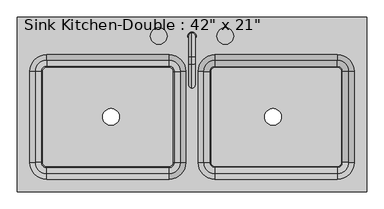
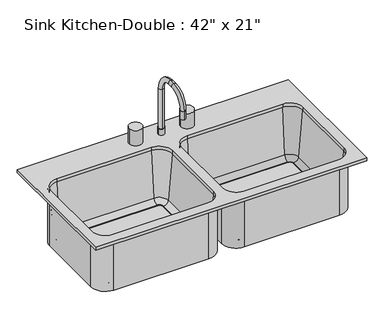
"""IFC4 building model written with IfcOpenShell, lengths in millimetres: flow terminal geometry."""

from ifc_helpers import new_model, si_unit, point, frame, frame_2d, origin, place, context, project, spatial, polyline, circle_curve, ellipse_curve, trimmed, segment, composite_curve, outline, extrude, source, transform, mapped, element, save
from ifc_brep_helpers import plane_surface, cylinder_surface, revolved_surface, advanced_brep


def flow_terminal_a53be723(model_context):
    return source(origin(), model_context, "Body", "SolidModel", [
        advanced_brep(
        [(2.9892406, 211.8954011, 927.1), (28.3892406, 211.8954011, 927.1), (15.6892406, 221.4204011, 1114.425), (15.6892406, 202.3704011, 1114.425), (15.6892406, 202.3704011, 952.5), (15.6892406, 221.4204011, 952.5), (15.6892406, 148.3954011, 1187.45), (15.6892406, 148.3954011, 1168.4), (15.6892406, 126.1704011, 1187.45), (15.6892406, 126.1704011, 1168.4), (15.6892406, 53.1454011, 1114.425), (15.6892406, 72.1954011, 1114.425), (15.6892406, 53.1454011, 1079.5), (15.6892406, 72.1954011, 1079.5), (2.9892406, 211.8954011, 952.5), (28.3892406, 211.8954011, 952.5)],
        [
            (0, 1, circle_curve(frame((15.6892406, 211.8954011, 927.1), z_axis=(0.0, 0.0, -1.0), x_axis=(1.0, 0.0, 0.0)), 12.7)),
            (1, 0, circle_curve(frame((15.6892406, 211.8954011, 927.1), z_axis=(0.0, 0.0, -1.0), x_axis=(1.0, 0.0, 0.0)), 12.7)),
            (2, 3, circle_curve(frame((15.6892406, 211.8954011, 1114.425), z_axis=(0.0, 0.0, -1.0), x_axis=(0.0, -1.0, 0.0)), 9.525)),
            (3, 4),
            (4, 5, circle_curve(frame((15.6892406, 211.8954011, 952.5), z_axis=(0.0, 0.0, 1.0), x_axis=(0.0, -1.0, 0.0)), 9.525)),
            (5, 2),
            (3, 2, circle_curve(frame((15.6892406, 211.8954011, 1114.425), z_axis=(0.0, 0.0, -1.0), x_axis=(0.0, -1.0, 0.0)), 9.525)),
            (5, 4, circle_curve(frame((15.6892406, 211.8954011, 952.5), z_axis=(0.0, 0.0, 1.0), x_axis=(0.0, -1.0, 0.0)), 9.525)),
            (2, 6, circle_curve(frame((15.6892406, 148.3954011, 1114.425), z_axis=(1.0, 0.0, 0.0), x_axis=(0.0, 1.0, 0.0)), 73.025)),
            (6, 7, circle_curve(frame((15.6892406, 148.3954011, 1177.925), z_axis=(0.0, 1.0, 0.0), x_axis=(0.0, 0.0, -1.0)), 9.525)),
            (7, 3, circle_curve(frame((15.6892406, 148.3954011, 1114.425), z_axis=(-1.0, 0.0, 0.0), x_axis=(0.0, 1.0, 0.0)), 53.975)),
            (7, 6, circle_curve(frame((15.6892406, 148.3954011, 1177.925), z_axis=(0.0, 1.0, 0.0), x_axis=(0.0, 0.0, -1.0)), 9.525)),
            (6, 8),
            (8, 9, circle_curve(frame((15.6892406, 126.1704011, 1177.925), z_axis=(0.0, 1.0, 0.0), x_axis=(0.0, 0.0, -1.0)), 9.525)),
            (9, 7),
            (9, 8, circle_curve(frame((15.6892406, 126.1704011, 1177.925), z_axis=(0.0, 1.0, 0.0), x_axis=(0.0, 0.0, -1.0)), 9.525)),
            (8, 10, circle_curve(frame((15.6892406, 126.1704011, 1114.425), z_axis=(1.0, 0.0, 0.0), x_axis=(0.0, 0.0, 1.0)), 73.025)),
            (10, 11, circle_curve(frame((15.6892406, 62.6704011, 1114.425), z_axis=(0.0, 0.0, 1.0), x_axis=(0.0, 1.0, 0.0)), 9.525)),
            (11, 9, circle_curve(frame((15.6892406, 126.1704011, 1114.425), z_axis=(-1.0, 0.0, 0.0), x_axis=(0.0, 0.0, 1.0)), 53.975)),
            (11, 10, circle_curve(frame((15.6892406, 62.6704011, 1114.425), z_axis=(0.0, 0.0, 1.0), x_axis=(0.0, 1.0, 0.0)), 9.525)),
            (12, 13, circle_curve(frame((15.6892406, 62.6704011, 1079.5), z_axis=(0.0, 0.0, -1.0), x_axis=(0.0, 1.0, 0.0)), 9.525)),
            (13, 12, circle_curve(frame((15.6892406, 62.6704011, 1079.5), z_axis=(0.0, 0.0, -1.0), x_axis=(0.0, 1.0, 0.0)), 9.525)),
            (10, 12),
            (13, 11),
            (14, 15, circle_curve(frame((15.6892406, 211.8954011, 952.5), z_axis=(0.0, 0.0, 1.0), x_axis=(1.0, 0.0, 0.0)), 12.7)),
            (15, 14, circle_curve(frame((15.6892406, 211.8954011, 952.5), z_axis=(0.0, 0.0, 1.0), x_axis=(1.0, 0.0, 0.0)), 12.7)),
            (14, 0),
            (1, 15),
        ],
        [
            plane_surface(frame((15.6892406, 202.3704011, 927.1), z_axis=(0.0, 0.0, -1.0), x_axis=(1.0, 0.0, 0.0))),
            cylinder_surface(frame((15.6892406, 211.8954011, 927.1), z_axis=(0.0, 0.0, -1.0), x_axis=(0.0, -1.0, 0.0)), 9.525),
            revolved_surface(trimmed(ellipse_curve(frame((15.6892406, 211.8954011, 1114.425), z_axis=(0.0, 0.0, -1.0), x_axis=(0.0, -1.0, 0.0)), 9.525, 9.525), [point((15.6892406, 221.4204011, 1114.425))], [point((15.6892406, 202.3704011, 1114.425))], True, "CARTESIAN"), (15.6892406, 148.3954011, 1114.425), (1.0, 0.0, 0.0)),
            revolved_surface(trimmed(ellipse_curve(frame((15.6892406, 211.8954011, 1114.425), z_axis=(0.0, 0.0, -1.0), x_axis=(0.0, -1.0, 0.0)), 9.525, 9.525), [point((15.6892406, 202.3704011, 1114.425))], [point((15.6892406, 221.4204011, 1114.425))], True, "CARTESIAN"), (15.6892406, 148.3954011, 1114.425), (1.0, 0.0, 0.0)),
            cylinder_surface(frame((15.6892406, 148.3954011, 1177.925), z_axis=(0.0, 1.0, 0.0), x_axis=(0.0, 0.0, -1.0)), 9.525),
            revolved_surface(trimmed(ellipse_curve(frame((15.6892406, 126.1704011, 1177.925), z_axis=(0.0, 1.0, 0.0), x_axis=(0.0, 0.0, -1.0)), 9.525, 9.525), [point((15.6892406, 126.1704011, 1187.45))], [point((15.6892406, 126.1704011, 1168.4))], True, "CARTESIAN"), (15.6892406, 126.1704011, 1114.425), (1.0, 0.0, 0.0)),
            revolved_surface(trimmed(ellipse_curve(frame((15.6892406, 126.1704011, 1177.925), z_axis=(0.0, 1.0, 0.0), x_axis=(0.0, 0.0, -1.0)), 9.525, 9.525), [point((15.6892406, 126.1704011, 1168.4))], [point((15.6892406, 126.1704011, 1187.45))], True, "CARTESIAN"), (15.6892406, 126.1704011, 1114.425), (1.0, 0.0, 0.0)),
            plane_surface(frame((15.6892406, 53.1454011, 1079.5), z_axis=(0.0, 0.0, -1.0), x_axis=(-1.0, 0.0, 0.0))),
            cylinder_surface(frame((15.6892406, 62.6704011, 1114.425), z_axis=(0.0, 0.0, 1.0), x_axis=(0.0, 1.0, 0.0)), 9.525),
            plane_surface(frame((28.3892406, 211.8954011, 952.5), z_axis=(0.0, 0.0, 1.0), x_axis=(0.0, 1.0, 0.0))),
            cylinder_surface(frame((15.6892406, 211.8954011, 927.1), z_axis=(0.0, 0.0, 1.0), x_axis=(1.0, 0.0, 0.0)), 12.7),
        ],
        [
            (0, [[1, 2]]),
            (1, [[3, 4, 5, 6]]),
            (1, [[7, -6, 8, -4]]),
            (2, [[-3, 9, 10, 11]]),
            (3, [[-7, -11, 12, -9]]),
            (4, [[-10, 13, 14, 15]]),
            (4, [[-12, -15, 16, -13]]),
            (5, [[-14, 17, 18, 19]]),
            (6, [[-16, -19, 20, -17]]),
            (7, [[21, 22]]),
            (8, [[-18, 23, -22, 24]]),
            (8, [[-20, -24, -21, -23]]),
            (9, [[25, 26], [-5, -8]]),
            (10, [[-25, 27, -2, 28]]),
            (10, [[-26, -28, -1, -27]]),
        ],
    ),
        advanced_brep(
        [(549.0892406, 269.0454011, 927.1), (-517.7107594, 269.0454011, 927.1), (-517.7107594, -264.3545989, 927.1), (549.0892406, -264.3545989, 927.1), (-54.1607594, 154.7454011, 927.1), (-3.3607594, 103.9454011, 927.1), (-3.3607594, -175.4545989, 927.1), (-54.1607594, -226.2545989, 927.1), (-428.8107594, -226.2545989, 927.1), (-479.6107594, -175.4545989, 927.1), (-479.6107594, 103.9454011, 927.1), (-428.8107594, 154.7454011, 927.1), (85.5392406, -226.2545989, 927.1), (34.7392406, -175.4545989, 927.1), (34.7392406, 103.9454011, 927.1), (85.5392406, 154.7454011, 927.1), (460.1892406, 154.7454011, 927.1), (510.9892406, 103.9454011, 927.1), (510.9892406, -175.4545989, 927.1), (460.1892406, -226.2545989, 927.1), (549.0892406, 269.0454011, 914.4), (549.0892406, -264.3545989, 914.4), (-517.7107594, -264.3545989, 914.4), (-517.7107594, 269.0454011, 914.4), (85.5392406, 161.0954011, 914.4), (28.3892406, 103.9454011, 914.4), (28.3892406, -175.4545989, 914.4), (85.5392406, -232.6045989, 914.4), (460.1892406, -232.6045989, 914.4), (517.3392406, -175.4545989, 914.4), (517.3392406, 103.9454011, 914.4), (460.1892406, 161.0954011, 914.4), (2.9892406, 103.9454011, 914.4), (-54.1607594, 161.0954011, 914.4), (-428.8107594, 161.0954011, 914.4), (-485.9607594, 103.9454011, 914.4), (-485.9607594, -175.4545989, 914.4), (-428.8107594, -232.6045989, 914.4), (-54.1607594, -232.6045989, 914.4), (2.9892406, -175.4545989, 914.4), (-54.1607594, 154.7454011, 914.4), (-3.3607594, 103.9454011, 914.4), (-3.3607594, -175.4545989, 914.4), (-54.1607594, -226.2545989, 914.4), (-428.8107594, -226.2545989, 914.4), (-479.6107594, -175.4545989, 914.4), (-479.6107594, 103.9454011, 914.4), (-428.8107594, 154.7454011, 914.4), (85.5392406, -226.2545989, 914.4), (34.7392406, -175.4545989, 914.4), (34.7392406, 103.9454011, 914.4), (85.5392406, 154.7454011, 914.4), (460.1892406, 154.7454011, 914.4), (510.9892406, 103.9454011, 914.4), (510.9892406, -175.4545989, 914.4), (460.1892406, -226.2545989, 914.4), (51.2733134, 103.9454011, 725.4146831), (85.5392406, 138.2113283, 725.4146831), (70.2508224, 103.9454011, 708.025), (85.5392406, 119.2338193, 708.025), (72.8392406, 103.9454011, 708.025), (85.5392406, 116.6454011, 708.025), (72.8392406, 103.9454011, 698.5), (85.5392406, 116.6454011, 698.5), (28.3892406, 103.9454011, 698.5), (85.5392406, 161.0954011, 698.5), (51.2733134, -175.4545989, 725.4146831), (70.2508224, -175.4545989, 708.025), (72.8392406, -175.4545989, 708.025), (72.8392406, -175.4545989, 698.5), (28.3892406, -175.4545989, 698.5), (85.5392406, -209.7205261, 725.4146831), (85.5392406, -190.7430171, 708.025), (85.5392406, -188.1545989, 708.025), (85.5392406, -188.1545989, 698.5), (85.5392406, -232.6045989, 698.5), (460.1892406, -209.7205261, 725.4146831), (460.1892406, -190.7430171, 708.025), (460.1892406, -188.1545989, 708.025), (460.1892406, -188.1545989, 698.5), (460.1892406, -232.6045989, 698.5), (494.4551678, -175.4545989, 725.4146831), (475.4776588, -175.4545989, 708.025), (472.8892406, -175.4545989, 708.025), (472.8892406, -175.4545989, 698.5), (517.3392406, -175.4545989, 698.5), (494.4551678, 103.9454011, 725.4146831), (475.4776588, 103.9454011, 708.025), (472.8892406, 103.9454011, 708.025), (472.8892406, 103.9454011, 698.5), (517.3392406, 103.9454011, 698.5), (460.1892406, 138.2113283, 725.4146831), (460.1892406, 119.2338193, 708.025), (460.1892406, 116.6454011, 708.025), (460.1892406, 116.6454011, 698.5), (460.1892406, 161.0954011, 698.5), (2.9892406, 103.9454011, 698.5), (-54.1607594, 161.0954011, 698.5), (-41.4607594, 103.9454011, 698.5), (-54.1607594, 116.6454011, 698.5), (-41.4607594, 103.9454011, 708.025), (-54.1607594, 116.6454011, 708.025), (-38.8723412, 103.9454011, 708.025), (-54.1607594, 119.2338193, 708.025), (-19.8948322, 103.9454011, 725.4146831), (-54.1607594, 138.2113283, 725.4146831), (2.9892406, -175.4545989, 698.5), (-41.4607594, -175.4545989, 698.5), (-41.4607594, -175.4545989, 708.025), (-38.8723412, -175.4545989, 708.025), (-19.8948322, -175.4545989, 725.4146831), (-54.1607594, -232.6045989, 698.5), (-54.1607594, -188.1545989, 698.5), (-54.1607594, -188.1545989, 708.025), (-54.1607594, -190.7430171, 708.025), (-54.1607594, -209.7205261, 725.4146831), (-428.8107594, -232.6045989, 698.5), (-428.8107594, -188.1545989, 698.5), (-428.8107594, -188.1545989, 708.025), (-428.8107594, -190.7430171, 708.025), (-428.8107594, -209.7205261, 725.4146831), (-485.9607594, -175.4545989, 698.5), (-441.5107594, -175.4545989, 698.5), (-441.5107594, -175.4545989, 708.025), (-444.0991776, -175.4545989, 708.025), (-463.0766866, -175.4545989, 725.4146831), (-485.9607594, 103.9454011, 698.5), (-441.5107594, 103.9454011, 698.5), (-441.5107594, 103.9454011, 708.025), (-444.0991776, 103.9454011, 708.025), (-463.0766866, 103.9454011, 725.4146831), (-428.8107594, 161.0954011, 698.5), (-428.8107594, 116.6454011, 698.5), (-428.8107594, 116.6454011, 708.025), (-428.8107594, 119.2338193, 708.025), (-428.8107594, 138.2113283, 725.4146831)],
        [
            (0, 1),
            (1, 2),
            (2, 3),
            (3, 0),
            (4, 5, circle_curve(frame((-54.1607594, 103.9454011, 927.1), z_axis=(0.0, 0.0, -1.0), x_axis=(1.0, 0.0, 0.0)), 50.8)),
            (5, 6),
            (6, 7, circle_curve(frame((-54.1607594, -175.4545989, 927.1), z_axis=(0.0, 0.0, -1.0), x_axis=(1.0, 0.0, 0.0)), 50.8)),
            (7, 8),
            (8, 9, circle_curve(frame((-428.8107594, -175.4545989, 927.1), z_axis=(0.0, 0.0, -1.0), x_axis=(1.0, 0.0, 0.0)), 50.8)),
            (9, 10),
            (10, 11, circle_curve(frame((-428.8107594, 103.9454011, 927.1), z_axis=(0.0, 0.0, -1.0), x_axis=(1.0, 0.0, 0.0)), 50.8)),
            (11, 4),
            (12, 13, circle_curve(frame((85.5392406, -175.4545989, 927.1), z_axis=(0.0, 0.0, -1.0), x_axis=(1.0, 0.0, 0.0)), 50.8)),
            (13, 14),
            (14, 15, circle_curve(frame((85.5392406, 103.9454011, 927.1), z_axis=(0.0, 0.0, -1.0), x_axis=(1.0, 0.0, 0.0)), 50.8)),
            (15, 16),
            (16, 17, circle_curve(frame((460.1892406, 103.9454011, 927.1), z_axis=(0.0, 0.0, -1.0), x_axis=(1.0, 0.0, 0.0)), 50.8)),
            (17, 18),
            (18, 19, circle_curve(frame((460.1892406, -175.4545989, 927.1), z_axis=(0.0, 0.0, -1.0), x_axis=(1.0, 0.0, 0.0)), 50.8)),
            (19, 12),
            (20, 21),
            (21, 22),
            (22, 23),
            (23, 20),
            (24, 25, circle_curve(frame((85.5392406, 103.9454011, 914.4), z_axis=(0.0, 0.0, 1.0), x_axis=(0.0, 1.0, 0.0)), 57.15)),
            (25, 26),
            (26, 27, circle_curve(frame((85.5392406, -175.4545989, 914.4), z_axis=(0.0, 0.0, 1.0), x_axis=(-1.0, 0.0, 0.0)), 57.15)),
            (27, 28),
            (28, 29, circle_curve(frame((460.1892406, -175.4545989, 914.4), z_axis=(0.0, 0.0, 1.0), x_axis=(0.0, -1.0, 0.0)), 57.15)),
            (29, 30),
            (30, 31, circle_curve(frame((460.1892406, 103.9454011, 914.4), z_axis=(0.0, 0.0, 1.0), x_axis=(1.0, 0.0, 0.0)), 57.15)),
            (31, 24),
            (32, 33, circle_curve(frame((-54.1607594, 103.9454011, 914.4), z_axis=(0.0, 0.0, 1.0), x_axis=(0.0, 1.0, 0.0)), 57.15)),
            (33, 34),
            (34, 35, circle_curve(frame((-428.8107594, 103.9454011, 914.4), z_axis=(0.0, 0.0, 1.0), x_axis=(-1.0, 0.0, 0.0)), 57.15)),
            (35, 36),
            (36, 37, circle_curve(frame((-428.8107594, -175.4545989, 914.4), z_axis=(0.0, 0.0, 1.0), x_axis=(0.0, -1.0, 0.0)), 57.15)),
            (37, 38),
            (38, 39, circle_curve(frame((-54.1607594, -175.4545989, 914.4), z_axis=(0.0, 0.0, 1.0), x_axis=(1.0, 0.0, 0.0)), 57.15)),
            (39, 32),
            (0, 20),
            (23, 1),
            (22, 2),
            (21, 3),
            (4, 40),
            (40, 41, circle_curve(frame((-54.1607594, 103.9454011, 914.4), z_axis=(0.0, 0.0, -1.0), x_axis=(1.0, 0.0, 0.0)), 50.8)),
            (41, 5),
            (41, 42),
            (42, 6),
            (42, 43, circle_curve(frame((-54.1607594, -175.4545989, 914.4), z_axis=(0.0, 0.0, -1.0), x_axis=(1.0, 0.0, 0.0)), 50.8)),
            (43, 7),
            (43, 44),
            (44, 8),
            (44, 45, circle_curve(frame((-428.8107594, -175.4545989, 914.4), z_axis=(0.0, 0.0, -1.0), x_axis=(1.0, 0.0, 0.0)), 50.8)),
            (45, 9),
            (45, 46),
            (46, 10),
            (46, 47, circle_curve(frame((-428.8107594, 103.9454011, 914.4), z_axis=(0.0, 0.0, -1.0), x_axis=(1.0, 0.0, 0.0)), 50.8)),
            (47, 11),
            (47, 40),
            (12, 48),
            (48, 49, circle_curve(frame((85.5392406, -175.4545989, 914.4), z_axis=(0.0, 0.0, -1.0), x_axis=(1.0, 0.0, 0.0)), 50.8)),
            (49, 13),
            (49, 50),
            (50, 14),
            (50, 51, circle_curve(frame((85.5392406, 103.9454011, 914.4), z_axis=(0.0, 0.0, -1.0), x_axis=(1.0, 0.0, 0.0)), 50.8)),
            (51, 15),
            (51, 52),
            (52, 16),
            (52, 53, circle_curve(frame((460.1892406, 103.9454011, 914.4), z_axis=(0.0, 0.0, -1.0), x_axis=(1.0, 0.0, 0.0)), 50.8)),
            (53, 17),
            (53, 54),
            (54, 18),
            (54, 55, circle_curve(frame((460.1892406, -175.4545989, 914.4), z_axis=(0.0, 0.0, -1.0), x_axis=(1.0, 0.0, 0.0)), 50.8)),
            (55, 19),
            (55, 48),
            (56, 57, circle_curve(frame((85.5392406, 103.9454011, 725.4146831), z_axis=(0.0, 0.0, -1.0), x_axis=(0.0, 1.0, 0.0)), 34.2659272)),
            (57, 51),
            (50, 56),
            (56, 58, circle_curve(frame((70.2508224, 103.9454011, 727.075), z_axis=(0.0, -1.0, 0.0), x_axis=(1.0, 0.0, 0.0)), 19.05)),
            (58, 59, circle_curve(frame((85.5392406, 103.9454011, 708.025), z_axis=(0.0, 0.0, -1.0), x_axis=(0.0, 1.0, 0.0)), 15.2884182)),
            (59, 57, circle_curve(frame((85.5392406, 119.2338193, 727.075), z_axis=(1.0, 0.0, 0.0), x_axis=(0.0, -1.0, 0.0)), 19.05)),
            (58, 60),
            (60, 61, circle_curve(frame((85.5392406, 103.9454011, 708.025), z_axis=(0.0, 0.0, -1.0), x_axis=(0.0, 1.0, 0.0)), 12.7)),
            (61, 59),
            (60, 62),
            (62, 63, circle_curve(frame((85.5392406, 103.9454011, 698.5), z_axis=(0.0, 0.0, -1.0), x_axis=(0.0, 1.0, 0.0)), 12.7)),
            (63, 61),
            (62, 64),
            (64, 65, circle_curve(frame((85.5392406, 103.9454011, 698.5), z_axis=(0.0, 0.0, -1.0), x_axis=(0.0, 1.0, 0.0)), 57.15)),
            (65, 63),
            (64, 25),
            (24, 65),
            (49, 66),
            (66, 56),
            (66, 67, circle_curve(frame((70.2508224, -175.4545989, 727.075), z_axis=(0.0, -1.0, 0.0), x_axis=(1.0, 0.0, 0.0)), 19.05)),
            (67, 58),
            (67, 68),
            (68, 60),
            (68, 69),
            (69, 62),
            (69, 70),
            (70, 64),
            (70, 26),
            (48, 71),
            (71, 66, circle_curve(frame((85.5392406, -175.4545989, 725.4146831), z_axis=(0.0, 0.0, -1.0), x_axis=(-1.0, 0.0, 0.0)), 34.2659272)),
            (71, 72, circle_curve(frame((85.5392406, -190.7430171, 727.075), z_axis=(1.0, 0.0, 0.0), x_axis=(0.0, 1.0, 0.0)), 19.05)),
            (72, 67, circle_curve(frame((85.5392406, -175.4545989, 708.025), z_axis=(0.0, 0.0, -1.0), x_axis=(-1.0, 0.0, 0.0)), 15.2884182)),
            (72, 73),
            (73, 68, circle_curve(frame((85.5392406, -175.4545989, 708.025), z_axis=(0.0, 0.0, -1.0), x_axis=(-1.0, 0.0, 0.0)), 12.7)),
            (73, 74),
            (74, 69, circle_curve(frame((85.5392406, -175.4545989, 698.5), z_axis=(0.0, 0.0, -1.0), x_axis=(-1.0, 0.0, 0.0)), 12.7)),
            (74, 75),
            (75, 70, circle_curve(frame((85.5392406, -175.4545989, 698.5), z_axis=(0.0, 0.0, -1.0), x_axis=(-1.0, 0.0, 0.0)), 57.15)),
            (75, 27),
            (55, 76),
            (76, 71),
            (76, 77, circle_curve(frame((460.1892406, -190.7430171, 727.075), z_axis=(1.0, 0.0, 0.0), x_axis=(0.0, 1.0, 0.0)), 19.05)),
            (77, 72),
            (77, 78),
            (78, 73),
            (78, 79),
            (79, 74),
            (79, 80),
            (80, 75),
            (80, 28),
            (54, 81),
            (81, 76, circle_curve(frame((460.1892406, -175.4545989, 725.4146831), z_axis=(0.0, 0.0, -1.0), x_axis=(0.0, -1.0, 0.0)), 34.2659272)),
            (81, 82, circle_curve(frame((475.4776588, -175.4545989, 727.075), z_axis=(0.0, 1.0, 0.0), x_axis=(-1.0, 0.0, 0.0)), 19.05)),
            (82, 77, circle_curve(frame((460.1892406, -175.4545989, 708.025), z_axis=(0.0, 0.0, -1.0), x_axis=(0.0, -1.0, 0.0)), 15.2884182)),
            (82, 83),
            (83, 78, circle_curve(frame((460.1892406, -175.4545989, 708.025), z_axis=(0.0, 0.0, -1.0), x_axis=(0.0, -1.0, 0.0)), 12.7)),
            (83, 84),
            (84, 79, circle_curve(frame((460.1892406, -175.4545989, 698.5), z_axis=(0.0, 0.0, -1.0), x_axis=(0.0, -1.0, 0.0)), 12.7)),
            (84, 85),
            (85, 80, circle_curve(frame((460.1892406, -175.4545989, 698.5), z_axis=(0.0, 0.0, -1.0), x_axis=(0.0, -1.0, 0.0)), 57.15)),
            (85, 29),
            (53, 86),
            (86, 81),
            (86, 87, circle_curve(frame((475.4776588, 103.9454011, 727.075), z_axis=(0.0, 1.0, 0.0), x_axis=(-1.0, 0.0, 0.0)), 19.05)),
            (87, 82),
            (87, 88),
            (88, 83),
            (88, 89),
            (89, 84),
            (89, 90),
            (90, 85),
            (90, 30),
            (52, 91),
            (91, 86, circle_curve(frame((460.1892406, 103.9454011, 725.4146831), z_axis=(0.0, 0.0, -1.0), x_axis=(1.0, 0.0, 0.0)), 34.2659272)),
            (91, 92, circle_curve(frame((460.1892406, 119.2338193, 727.075), z_axis=(-1.0, 0.0, 0.0), x_axis=(0.0, -1.0, 0.0)), 19.05)),
            (92, 87, circle_curve(frame((460.1892406, 103.9454011, 708.025), z_axis=(0.0, 0.0, -1.0), x_axis=(1.0, 0.0, 0.0)), 15.2884182)),
            (92, 93),
            (93, 88, circle_curve(frame((460.1892406, 103.9454011, 708.025), z_axis=(0.0, 0.0, -1.0), x_axis=(1.0, 0.0, 0.0)), 12.7)),
            (93, 94),
            (94, 89, circle_curve(frame((460.1892406, 103.9454011, 698.5), z_axis=(0.0, 0.0, -1.0), x_axis=(1.0, 0.0, 0.0)), 12.7)),
            (94, 95),
            (95, 90, circle_curve(frame((460.1892406, 103.9454011, 698.5), z_axis=(0.0, 0.0, -1.0), x_axis=(1.0, 0.0, 0.0)), 57.15)),
            (95, 31),
            (57, 91),
            (59, 92),
            (61, 93),
            (63, 94),
            (65, 95),
            (96, 97, circle_curve(frame((-54.1607594, 103.9454011, 698.5), z_axis=(0.0, 0.0, 1.0), x_axis=(0.0, 1.0, 0.0)), 57.15)),
            (97, 33),
            (32, 96),
            (96, 98),
            (98, 99, circle_curve(frame((-54.1607594, 103.9454011, 698.5), z_axis=(0.0, 0.0, 1.0), x_axis=(0.0, 1.0, 0.0)), 12.7)),
            (99, 97),
            (98, 100),
            (100, 101, circle_curve(frame((-54.1607594, 103.9454011, 708.025), z_axis=(0.0, 0.0, 1.0), x_axis=(0.0, 1.0, 0.0)), 12.7)),
            (101, 99),
            (100, 102),
            (102, 103, circle_curve(frame((-54.1607594, 103.9454011, 708.025), z_axis=(0.0, 0.0, 1.0), x_axis=(0.0, 1.0, 0.0)), 15.2884182)),
            (103, 101),
            (102, 104, circle_curve(frame((-38.8723412, 103.9454011, 727.075), z_axis=(0.0, -1.0, 0.0), x_axis=(1.0, 0.0, 0.0)), 19.05)),
            (104, 105, circle_curve(frame((-54.1607594, 103.9454011, 725.4146831), z_axis=(0.0, 0.0, 1.0), x_axis=(0.0, 1.0, 0.0)), 34.2659272)),
            (105, 103, circle_curve(frame((-54.1607594, 119.2338193, 727.075), z_axis=(-1.0, 0.0, 0.0), x_axis=(0.0, 1.0, 0.0)), 19.05)),
            (104, 41),
            (40, 105),
            (39, 106),
            (106, 96),
            (106, 107),
            (107, 98),
            (107, 108),
            (108, 100),
            (108, 109),
            (109, 102),
            (109, 110, circle_curve(frame((-38.8723412, -175.4545989, 727.075), z_axis=(0.0, -1.0, 0.0), x_axis=(1.0, 0.0, 0.0)), 19.05)),
            (110, 104),
            (110, 42),
            (38, 111),
            (111, 106, circle_curve(frame((-54.1607594, -175.4545989, 698.5), z_axis=(0.0, 0.0, 1.0), x_axis=(1.0, 0.0, 0.0)), 57.15)),
            (111, 112),
            (112, 107, circle_curve(frame((-54.1607594, -175.4545989, 698.5), z_axis=(0.0, 0.0, 1.0), x_axis=(1.0, 0.0, 0.0)), 12.7)),
            (112, 113),
            (113, 108, circle_curve(frame((-54.1607594, -175.4545989, 708.025), z_axis=(0.0, 0.0, 1.0), x_axis=(1.0, 0.0, 0.0)), 12.7)),
            (113, 114),
            (114, 109, circle_curve(frame((-54.1607594, -175.4545989, 708.025), z_axis=(0.0, 0.0, 1.0), x_axis=(1.0, 0.0, 0.0)), 15.2884182)),
            (114, 115, circle_curve(frame((-54.1607594, -190.7430171, 727.075), z_axis=(-1.0, 0.0, 0.0), x_axis=(0.0, -1.0, 0.0)), 19.05)),
            (115, 110, circle_curve(frame((-54.1607594, -175.4545989, 725.4146831), z_axis=(0.0, 0.0, 1.0), x_axis=(1.0, 0.0, 0.0)), 34.2659272)),
            (115, 43),
            (37, 116),
            (116, 111),
            (116, 117),
            (117, 112),
            (117, 118),
            (118, 113),
            (118, 119),
            (119, 114),
            (119, 120, circle_curve(frame((-428.8107594, -190.7430171, 727.075), z_axis=(-1.0, 0.0, 0.0), x_axis=(0.0, -1.0, 0.0)), 19.05)),
            (120, 115),
            (120, 44),
            (36, 121),
            (121, 116, circle_curve(frame((-428.8107594, -175.4545989, 698.5), z_axis=(0.0, 0.0, 1.0), x_axis=(0.0, -1.0, 0.0)), 57.15)),
            (121, 122),
            (122, 117, circle_curve(frame((-428.8107594, -175.4545989, 698.5), z_axis=(0.0, 0.0, 1.0), x_axis=(0.0, -1.0, 0.0)), 12.7)),
            (122, 123),
            (123, 118, circle_curve(frame((-428.8107594, -175.4545989, 708.025), z_axis=(0.0, 0.0, 1.0), x_axis=(0.0, -1.0, 0.0)), 12.7)),
            (123, 124),
            (124, 119, circle_curve(frame((-428.8107594, -175.4545989, 708.025), z_axis=(0.0, 0.0, 1.0), x_axis=(0.0, -1.0, 0.0)), 15.2884182)),
            (124, 125, circle_curve(frame((-444.0991776, -175.4545989, 727.075), z_axis=(0.0, 1.0, 0.0), x_axis=(-1.0, 0.0, 0.0)), 19.05)),
            (125, 120, circle_curve(frame((-428.8107594, -175.4545989, 725.4146831), z_axis=(0.0, 0.0, 1.0), x_axis=(0.0, -1.0, 0.0)), 34.2659272)),
            (125, 45),
            (35, 126),
            (126, 121),
            (126, 127),
            (127, 122),
            (127, 128),
            (128, 123),
            (128, 129),
            (129, 124),
            (129, 130, circle_curve(frame((-444.0991776, 103.9454011, 727.075), z_axis=(0.0, 1.0, 0.0), x_axis=(-1.0, 0.0, 0.0)), 19.05)),
            (130, 125),
            (130, 46),
            (34, 131),
            (131, 126, circle_curve(frame((-428.8107594, 103.9454011, 698.5), z_axis=(0.0, 0.0, 1.0), x_axis=(-1.0, 0.0, 0.0)), 57.15)),
            (131, 132),
            (132, 127, circle_curve(frame((-428.8107594, 103.9454011, 698.5), z_axis=(0.0, 0.0, 1.0), x_axis=(-1.0, 0.0, 0.0)), 12.7)),
            (132, 133),
            (133, 128, circle_curve(frame((-428.8107594, 103.9454011, 708.025), z_axis=(0.0, 0.0, 1.0), x_axis=(-1.0, 0.0, 0.0)), 12.7)),
            (133, 134),
            (134, 129, circle_curve(frame((-428.8107594, 103.9454011, 708.025), z_axis=(0.0, 0.0, 1.0), x_axis=(-1.0, 0.0, 0.0)), 15.2884182)),
            (134, 135, circle_curve(frame((-428.8107594, 119.2338193, 727.075), z_axis=(1.0, 0.0, 0.0), x_axis=(0.0, 1.0, 0.0)), 19.05)),
            (135, 130, circle_curve(frame((-428.8107594, 103.9454011, 725.4146831), z_axis=(0.0, 0.0, 1.0), x_axis=(-1.0, 0.0, 0.0)), 34.2659272)),
            (135, 47),
            (97, 131),
            (99, 132),
            (101, 133),
            (103, 134),
            (105, 135),
        ],
        [
            plane_surface(frame((-517.7107594, 269.0454011, 927.1), z_axis=(0.0, 0.0, 1.0), x_axis=(-1.0, 0.0, 0.0))),
            plane_surface(frame((-517.7107594, 269.0454011, 914.4), z_axis=(0.0, 0.0, -1.0), x_axis=(1.0, 0.0, 0.0))),
            plane_surface(frame((549.0892406, 269.0454011, 927.1), z_axis=(0.0, 1.0, 0.0), x_axis=(0.0, 0.0, -1.0))),
            plane_surface(frame((-517.7107594, 269.0454011, 927.1), z_axis=(-1.0, 0.0, 0.0), x_axis=(0.0, 0.0, -1.0))),
            plane_surface(frame((-517.7107594, -264.3545989, 927.1), z_axis=(0.0, -1.0, 0.0), x_axis=(0.0, 0.0, -1.0))),
            plane_surface(frame((549.0892406, -264.3545989, 927.1), z_axis=(1.0, 0.0, 0.0), x_axis=(0.0, 0.0, -1.0))),
            revolved_surface(polyline([(-3.3607594000000063, 103.9454011, 914.4), (-3.3607594000000063, 103.9454011, 927.1)]), (-54.1607594, 103.9454011, 0.0), (0.0, 0.0, -1.0)),
            plane_surface(frame((-3.3607594, 103.9454011, 927.1), z_axis=(-1.0, 0.0, 0.0), x_axis=(0.0, 0.0, -1.0))),
            revolved_surface(polyline([(-3.3607594000000063, -175.4545989, 914.4), (-3.3607594000000063, -175.4545989, 927.1)]), (-54.1607594, -175.4545989, 0.0), (0.0, 0.0, -1.0)),
            plane_surface(frame((-54.1607594, -226.2545989, 927.1), z_axis=(0.0, 1.0, 0.0), x_axis=(0.0, 0.0, -1.0))),
            revolved_surface(polyline([(-378.0107594, -175.4545989, 914.4), (-378.0107594, -175.4545989, 927.1)]), (-428.8107594, -175.4545989, 0.0), (0.0, 0.0, -1.0)),
            plane_surface(frame((-479.6107594, -175.4545989, 927.1), z_axis=(1.0, 0.0, 0.0), x_axis=(0.0, 0.0, -1.0))),
            revolved_surface(polyline([(-378.0107594, 103.9454011, 914.4), (-378.0107594, 103.9454011, 927.1)]), (-428.8107594, 103.9454011, 0.0), (0.0, 0.0, -1.0)),
            plane_surface(frame((-428.8107594, 154.7454011, 927.1), z_axis=(0.0, -1.0, 0.0), x_axis=(0.0, 0.0, -1.0))),
            revolved_surface(polyline([(136.33924059999998, -175.4545989, 914.4), (136.33924059999998, -175.4545989, 927.1)]), (85.5392406, -175.4545989, 0.0), (0.0, 0.0, -1.0)),
            plane_surface(frame((34.7392406, -175.4545989, 927.1), z_axis=(1.0, 0.0, 0.0), x_axis=(0.0, 0.0, -1.0))),
            revolved_surface(polyline([(136.33924059999998, 103.9454011, 914.4), (136.33924059999998, 103.9454011, 927.1)]), (85.5392406, 103.9454011, 0.0), (0.0, 0.0, -1.0)),
            plane_surface(frame((85.5392406, 154.7454011, 927.1), z_axis=(0.0, -1.0, 0.0), x_axis=(0.0, 0.0, -1.0))),
            revolved_surface(polyline([(510.9892406, 103.9454011, 914.4), (510.9892406, 103.9454011, 927.1)]), (460.1892406, 103.9454011, 0.0), (0.0, 0.0, -1.0)),
            plane_surface(frame((510.9892406, 103.9454011, 927.1), z_axis=(-1.0, 0.0, 0.0), x_axis=(0.0, 0.0, -1.0))),
            revolved_surface(polyline([(510.9892406, -175.4545989, 914.4), (510.9892406, -175.4545989, 927.1)]), (460.1892406, -175.4545989, 0.0), (0.0, 0.0, -1.0)),
            plane_surface(frame((460.1892406, -226.2545989, 927.1), z_axis=(0.0, 1.0, 0.0), x_axis=(0.0, 0.0, -1.0))),
            revolved_surface(polyline([(85.5392406, 154.7454011, 914.4), (85.5392406, 138.2113283, 725.4146831)]), (85.5392406, 103.9454011, 0.0), (0.0, 0.0, 1.0)),
            revolved_surface(trimmed(ellipse_curve(frame((85.5392406, 119.2338193, 727.075), z_axis=(-1.0, 0.0, 0.0), x_axis=(0.0, -1.0, 0.0)), 19.05, 19.05), [point((85.5392406, 138.2113283, 725.4146831))], [point((85.5392406, 119.2338193, 708.025))], True, "CARTESIAN"), (85.5392406, 103.9454011, 0.0), (0.0, 0.0, 1.0)),
            plane_surface(frame((85.5392406, 103.9454011, 708.025), z_axis=(0.0, 0.0, 1.0), x_axis=(0.0, 1.0, 0.0))),
            revolved_surface(polyline([(85.5392406, 116.6454011, 708.025), (85.5392406, 116.6454011, 698.5)]), (85.5392406, 103.9454011, 0.0), (0.0, 0.0, 1.0)),
            plane_surface(frame((85.5392406, 103.9454011, 698.5), z_axis=(0.0, 0.0, -1.0), x_axis=(0.0, 1.0, 0.0))),
            cylinder_surface(frame((85.5392406, 103.9454011, 0.0), z_axis=(0.0, 0.0, 1.0), x_axis=(0.0, 1.0, 0.0)), 57.15),
            plane_surface(frame((34.7392406, 103.9454011, 914.4), z_axis=(0.996194698091745, 0.0, 0.08715574274766508), x_axis=(0.0, -1.0, 0.0))),
            revolved_surface(polyline([(89.3008224, -175.45459889999998, 727.075), (89.3008224, 103.9454011, 727.075)]), (70.2508224, 103.9454011, 727.075), (0.0, -1.0, 0.0)),
            plane_surface(frame((70.2508224, 103.9454011, 708.025), z_axis=(0.0, 0.0, 1.0), x_axis=(0.0, -1.0, 0.0))),
            plane_surface(frame((72.8392406, 103.9454011, 708.025), z_axis=(1.0, 0.0, 0.0), x_axis=(0.0, -1.0, 0.0))),
            plane_surface(frame((72.8392406, 103.9454011, 698.5), z_axis=(0.0, 0.0, -1.0), x_axis=(0.0, -1.0, 0.0))),
            plane_surface(frame((28.3892406, 103.9454011, 698.5), z_axis=(-1.0, 0.0, 0.0), x_axis=(0.0, -1.0, 0.0))),
            revolved_surface(polyline([(34.7392406, -175.4545989, 914.4), (51.2733134, -175.4545989, 725.4146831)]), (85.5392406, -175.4545989, 0.0), (0.0, 0.0, 1.0)),
            revolved_surface(trimmed(ellipse_curve(frame((70.2508224, -175.4545989, 727.075), z_axis=(0.0, -1.0, 0.0), x_axis=(1.0, 0.0, 0.0)), 19.05, 19.05), [point((51.2733134, -175.4545989, 725.4146831))], [point((70.2508224, -175.4545989, 708.025))], True, "CARTESIAN"), (85.5392406, -175.4545989, 0.0), (0.0, 0.0, 1.0)),
            plane_surface(frame((85.5392406, -175.4545989, 708.025), z_axis=(0.0, 0.0, 1.0), x_axis=(-1.0, 0.0, 0.0))),
            revolved_surface(polyline([(72.8392406, -175.4545989, 708.025), (72.8392406, -175.4545989, 698.5)]), (85.5392406, -175.4545989, 0.0), (0.0, 0.0, 1.0)),
            plane_surface(frame((85.5392406, -175.4545989, 698.5), z_axis=(0.0, 0.0, -1.0), x_axis=(-1.0, 0.0, 0.0))),
            cylinder_surface(frame((85.5392406, -175.4545989, 0.0), z_axis=(0.0, 0.0, 1.0), x_axis=(-1.0, 0.0, 0.0)), 57.15),
            plane_surface(frame((85.5392406, -226.2545989, 914.4), z_axis=(0.0, 0.996194698091745, 0.08715574274766508), x_axis=(1.0, 0.0, 0.0))),
            revolved_surface(polyline([(460.18924059999995, -171.6930171, 727.075), (85.5392406, -171.6930171, 727.075)]), (85.5392406, -190.7430171, 727.075), (1.0, 0.0, 0.0)),
            plane_surface(frame((85.5392406, -190.7430171, 708.025), z_axis=(0.0, 0.0, 1.0), x_axis=(1.0, 0.0, 0.0))),
            plane_surface(frame((85.5392406, -188.1545989, 708.025), z_axis=(0.0, 1.0, 0.0), x_axis=(1.0, 0.0, 0.0))),
            plane_surface(frame((85.5392406, -188.1545989, 698.5), z_axis=(0.0, 0.0, -1.0), x_axis=(1.0, 0.0, 0.0))),
            plane_surface(frame((85.5392406, -232.6045989, 698.5), z_axis=(0.0, -1.0, 0.0), x_axis=(1.0, 0.0, 0.0))),
            revolved_surface(polyline([(460.1892406, -226.2545989, 914.4), (460.1892406, -209.7205261, 725.4146831)]), (460.1892406, -175.4545989, 0.0), (0.0, 0.0, 1.0)),
            revolved_surface(trimmed(ellipse_curve(frame((460.1892406, -190.7430171, 727.075), z_axis=(1.0, 0.0, 0.0), x_axis=(0.0, 1.0, 0.0)), 19.05, 19.05), [point((460.1892406, -209.7205261, 725.4146831))], [point((460.1892406, -190.7430171, 708.025))], True, "CARTESIAN"), (460.1892406, -175.4545989, 0.0), (0.0, 0.0, 1.0)),
            plane_surface(frame((460.1892406, -175.4545989, 708.025), z_axis=(0.0, 0.0, 1.0), x_axis=(0.0, -1.0, 0.0))),
            revolved_surface(polyline([(460.1892406, -188.1545989, 708.025), (460.1892406, -188.1545989, 698.5)]), (460.1892406, -175.4545989, 0.0), (0.0, 0.0, 1.0)),
            plane_surface(frame((460.1892406, -175.4545989, 698.5), z_axis=(0.0, 0.0, -1.0), x_axis=(0.0, -1.0, 0.0))),
            cylinder_surface(frame((460.1892406, -175.4545989, 0.0), z_axis=(0.0, 0.0, 1.0), x_axis=(0.0, -1.0, 0.0)), 57.15),
            plane_surface(frame((510.9892406, -175.4545989, 914.4), z_axis=(-0.996194698091745, 0.0, 0.08715574274766508), x_axis=(0.0, 1.0, 0.0))),
            revolved_surface(polyline([(456.42765879999996, 103.94540109999997, 727.075), (456.42765879999996, -175.4545989, 727.075)]), (475.4776588, -175.4545989, 727.075), (0.0, 1.0, 0.0)),
            plane_surface(frame((475.4776588, -175.4545989, 708.025), z_axis=(0.0, 0.0, 1.0), x_axis=(0.0, 1.0, 0.0))),
            plane_surface(frame((472.8892406, -175.4545989, 708.025), z_axis=(-1.0, 0.0, 0.0), x_axis=(0.0, 1.0, 0.0))),
            plane_surface(frame((472.8892406, -175.4545989, 698.5), z_axis=(0.0, 0.0, -1.0), x_axis=(0.0, 1.0, 0.0))),
            plane_surface(frame((517.3392406, -175.4545989, 698.5), z_axis=(1.0, 0.0, 0.0), x_axis=(0.0, 1.0, 0.0))),
            revolved_surface(polyline([(510.9892406, 103.9454011, 914.4), (494.4551678, 103.9454011, 725.4146831)]), (460.1892406, 103.9454011, 0.0), (0.0, 0.0, 1.0)),
            revolved_surface(trimmed(ellipse_curve(frame((475.4776588, 103.9454011, 727.075), z_axis=(0.0, 1.0, 0.0), x_axis=(-1.0, 0.0, 0.0)), 19.05, 19.05), [point((494.4551678, 103.9454011, 725.4146831))], [point((475.4776588, 103.9454011, 708.025))], True, "CARTESIAN"), (460.1892406, 103.9454011, 0.0), (0.0, 0.0, 1.0)),
            plane_surface(frame((460.1892406, 103.9454011, 708.025), z_axis=(0.0, 0.0, 1.0), x_axis=(1.0, 0.0, 0.0))),
            revolved_surface(polyline([(472.8892406, 103.9454011, 708.025), (472.8892406, 103.9454011, 698.5)]), (460.1892406, 103.9454011, 0.0), (0.0, 0.0, 1.0)),
            plane_surface(frame((460.1892406, 103.9454011, 698.5), z_axis=(0.0, 0.0, -1.0), x_axis=(1.0, 0.0, 0.0))),
            cylinder_surface(frame((460.1892406, 103.9454011, 0.0), z_axis=(0.0, 0.0, 1.0), x_axis=(1.0, 0.0, 0.0)), 57.15),
            plane_surface(frame((460.1892406, 154.7454011, 914.4), z_axis=(0.0, -0.996194698091745, 0.08715574274766508), x_axis=(-1.0, 0.0, 0.0))),
            revolved_surface(polyline([(85.53924060000003, 100.1838193, 727.075), (460.1892406, 100.1838193, 727.075)]), (460.1892406, 119.2338193, 727.075), (-1.0, 0.0, 0.0)),
            plane_surface(frame((460.1892406, 119.2338193, 708.025), z_axis=(0.0, 0.0, 1.0), x_axis=(-1.0, 0.0, 0.0))),
            plane_surface(frame((460.1892406, 116.6454011, 708.025), z_axis=(0.0, -1.0, 0.0), x_axis=(-1.0, 0.0, 0.0))),
            plane_surface(frame((460.1892406, 116.6454011, 698.5), z_axis=(0.0, 0.0, -1.0), x_axis=(-1.0, 0.0, 0.0))),
            plane_surface(frame((460.1892406, 161.0954011, 698.5), z_axis=(0.0, 1.0, 0.0), x_axis=(-1.0, 0.0, 0.0))),
            cylinder_surface(frame((-54.1607594, 103.9454011, 0.0), z_axis=(0.0, 0.0, -1.0), x_axis=(0.0, 1.0, 0.0)), 57.15),
            plane_surface(frame((-54.1607594, 103.9454011, 698.5), z_axis=(0.0, 0.0, -1.0), x_axis=(0.0, 1.0, 0.0))),
            revolved_surface(polyline([(-54.1607594, 116.6454011, 698.5), (-54.1607594, 116.6454011, 708.025)]), (-54.1607594, 103.9454011, 0.0), (0.0, 0.0, -1.0)),
            plane_surface(frame((-54.1607594, 103.9454011, 708.025), z_axis=(0.0, 0.0, 1.0), x_axis=(0.0, 1.0, 0.0))),
            revolved_surface(trimmed(ellipse_curve(frame((-54.1607594, 119.2338193, 727.075), z_axis=(1.0, 0.0, 0.0), x_axis=(0.0, 1.0, 0.0)), 19.05, 19.05), [point((-54.1607594, 119.2338193, 708.025))], [point((-54.1607594, 138.2113283, 725.4146831))], True, "CARTESIAN"), (-54.1607594, 103.9454011, 0.0), (0.0, 0.0, -1.0)),
            revolved_surface(polyline([(-54.1607594, 138.2113283, 725.4146831), (-54.1607594, 154.7454011, 914.4)]), (-54.1607594, 103.9454011, 0.0), (0.0, 0.0, -1.0)),
            plane_surface(frame((2.9892406, 103.9454011, 914.4), z_axis=(1.0, 0.0, 0.0), x_axis=(0.0, -1.0, 0.0))),
            plane_surface(frame((2.9892406, 103.9454011, 698.5), z_axis=(0.0, 0.0, -1.0), x_axis=(0.0, -1.0, 0.0))),
            plane_surface(frame((-41.4607594, 103.9454011, 698.5), z_axis=(-1.0, 0.0, 0.0), x_axis=(0.0, -1.0, 0.0))),
            plane_surface(frame((-41.4607594, 103.9454011, 708.025), z_axis=(0.0, 0.0, 1.0), x_axis=(0.0, -1.0, 0.0))),
            revolved_surface(polyline([(-19.8223412, -175.45459889999998, 727.075), (-19.8223412, 103.9454011, 727.075)]), (-38.8723412, 103.9454011, 727.075), (0.0, -1.0, 0.0)),
            plane_surface(frame((-19.8948322, 103.9454011, 725.4146831), z_axis=(-0.9961946980917439, 0.0, 0.08715574274767722), x_axis=(0.0, -1.0, 0.0))),
            cylinder_surface(frame((-54.1607594, -175.4545989, 0.0), z_axis=(0.0, 0.0, -1.0), x_axis=(1.0, 0.0, 0.0)), 57.15),
            plane_surface(frame((-54.1607594, -175.4545989, 698.5), z_axis=(0.0, 0.0, -1.0), x_axis=(1.0, 0.0, 0.0))),
            revolved_surface(polyline([(-41.4607594, -175.4545989, 698.5), (-41.4607594, -175.4545989, 708.025)]), (-54.1607594, -175.4545989, 0.0), (0.0, 0.0, -1.0)),
            plane_surface(frame((-54.1607594, -175.4545989, 708.025), z_axis=(0.0, 0.0, 1.0), x_axis=(1.0, 0.0, 0.0))),
            revolved_surface(trimmed(ellipse_curve(frame((-38.8723412, -175.4545989, 727.075), z_axis=(0.0, -1.0, 0.0), x_axis=(1.0, 0.0, 0.0)), 19.05, 19.05), [point((-38.8723412, -175.4545989, 708.025))], [point((-19.8948322, -175.4545989, 725.4146831))], True, "CARTESIAN"), (-54.1607594, -175.4545989, 0.0), (0.0, 0.0, -1.0)),
            revolved_surface(polyline([(-19.8948322, -175.4545989, 725.4146831), (-3.3607594, -175.4545989, 914.4)]), (-54.1607594, -175.4545989, 0.0), (0.0, 0.0, -1.0)),
            plane_surface(frame((-54.1607594, -232.6045989, 914.4), z_axis=(0.0, -1.0, 0.0), x_axis=(-1.0, 0.0, 0.0))),
            plane_surface(frame((-54.1607594, -232.6045989, 698.5), z_axis=(0.0, 0.0, -1.0), x_axis=(-1.0, 0.0, 0.0))),
            plane_surface(frame((-54.1607594, -188.1545989, 698.5), z_axis=(0.0, 1.0, 0.0), x_axis=(-1.0, 0.0, 0.0))),
            plane_surface(frame((-54.1607594, -188.1545989, 708.025), z_axis=(0.0, 0.0, 1.0), x_axis=(-1.0, 0.0, 0.0))),
            revolved_surface(polyline([(-428.8107594, -209.79301710000001, 727.075), (-54.1607594, -209.79301710000001, 727.075)]), (-54.1607594, -190.7430171, 727.075), (-1.0, 0.0, 0.0)),
            plane_surface(frame((-54.1607594, -209.7205261, 725.4146831), z_axis=(0.0, 0.9961946980917439, 0.08715574274767722), x_axis=(-1.0, 0.0, 0.0))),
            cylinder_surface(frame((-428.8107594, -175.4545989, 0.0), z_axis=(0.0, 0.0, -1.0), x_axis=(0.0, -1.0, 0.0)), 57.15),
            plane_surface(frame((-428.8107594, -175.4545989, 698.5), z_axis=(0.0, 0.0, -1.0), x_axis=(0.0, -1.0, 0.0))),
            revolved_surface(polyline([(-428.8107594, -188.1545989, 698.5), (-428.8107594, -188.1545989, 708.025)]), (-428.8107594, -175.4545989, 0.0), (0.0, 0.0, -1.0)),
            plane_surface(frame((-428.8107594, -175.4545989, 708.025), z_axis=(0.0, 0.0, 1.0), x_axis=(0.0, -1.0, 0.0))),
            revolved_surface(trimmed(ellipse_curve(frame((-428.8107594, -190.7430171, 727.075), z_axis=(-1.0, 0.0, 0.0), x_axis=(0.0, -1.0, 0.0)), 19.05, 19.05), [point((-428.8107594, -190.7430171, 708.025))], [point((-428.8107594, -209.7205261, 725.4146831))], True, "CARTESIAN"), (-428.8107594, -175.4545989, 0.0), (0.0, 0.0, -1.0)),
            revolved_surface(polyline([(-428.8107594, -209.7205261, 725.4146831), (-428.8107594, -226.2545989, 914.4)]), (-428.8107594, -175.4545989, 0.0), (0.0, 0.0, -1.0)),
            plane_surface(frame((-485.9607594, -175.4545989, 914.4), z_axis=(-1.0, 0.0, 0.0), x_axis=(0.0, 1.0, 0.0))),
            plane_surface(frame((-485.9607594, -175.4545989, 698.5), z_axis=(0.0, 0.0, -1.0), x_axis=(0.0, 1.0, 0.0))),
            plane_surface(frame((-441.5107594, -175.4545989, 698.5), z_axis=(1.0, 0.0, 0.0), x_axis=(0.0, 1.0, 0.0))),
            plane_surface(frame((-441.5107594, -175.4545989, 708.025), z_axis=(0.0, 0.0, 1.0), x_axis=(0.0, 1.0, 0.0))),
            revolved_surface(polyline([(-463.14917760000003, 103.94540109999997, 727.075), (-463.14917760000003, -175.4545989, 727.075)]), (-444.0991776, -175.4545989, 727.075), (0.0, 1.0, 0.0)),
            plane_surface(frame((-463.0766866, -175.4545989, 725.4146831), z_axis=(0.9961946980917439, 0.0, 0.08715574274767722), x_axis=(0.0, 1.0, 0.0))),
            cylinder_surface(frame((-428.8107594, 103.9454011, 0.0), z_axis=(0.0, 0.0, -1.0), x_axis=(-1.0, 0.0, 0.0)), 57.15),
            plane_surface(frame((-428.8107594, 103.9454011, 698.5), z_axis=(0.0, 0.0, -1.0), x_axis=(-1.0, 0.0, 0.0))),
            revolved_surface(polyline([(-441.5107594, 103.9454011, 698.5), (-441.5107594, 103.9454011, 708.025)]), (-428.8107594, 103.9454011, 0.0), (0.0, 0.0, -1.0)),
            plane_surface(frame((-428.8107594, 103.9454011, 708.025), z_axis=(0.0, 0.0, 1.0), x_axis=(-1.0, 0.0, 0.0))),
            revolved_surface(trimmed(ellipse_curve(frame((-444.0991776, 103.9454011, 727.075), z_axis=(0.0, 1.0, 0.0), x_axis=(-1.0, 0.0, 0.0)), 19.05, 19.05), [point((-444.0991776, 103.9454011, 708.025))], [point((-463.0766866, 103.9454011, 725.4146831))], True, "CARTESIAN"), (-428.8107594, 103.9454011, 0.0), (0.0, 0.0, -1.0)),
            revolved_surface(polyline([(-463.0766866, 103.9454011, 725.4146831), (-479.6107594, 103.9454011, 914.4)]), (-428.8107594, 103.9454011, 0.0), (0.0, 0.0, -1.0)),
            plane_surface(frame((-428.8107594, 161.0954011, 914.4), z_axis=(0.0, 1.0, 0.0), x_axis=(1.0, 0.0, 0.0))),
            plane_surface(frame((-428.8107594, 161.0954011, 698.5), z_axis=(0.0, 0.0, -1.0), x_axis=(1.0, 0.0, 0.0))),
            plane_surface(frame((-428.8107594, 116.6454011, 698.5), z_axis=(0.0, -1.0, 0.0), x_axis=(1.0, 0.0, 0.0))),
            plane_surface(frame((-428.8107594, 116.6454011, 708.025), z_axis=(0.0, 0.0, 1.0), x_axis=(1.0, 0.0, 0.0))),
            revolved_surface(polyline([(-54.16075940000002, 138.2838193, 727.075), (-428.8107594, 138.2838193, 727.075)]), (-428.8107594, 119.2338193, 727.075), (1.0, 0.0, 0.0)),
            plane_surface(frame((-428.8107594, 138.2113283, 725.4146831), z_axis=(0.0, -0.9961946980917439, 0.08715574274767722), x_axis=(1.0, 0.0, 0.0))),
        ],
        [
            (0, [[1, 2, 3, 4], [5, 6, 7, 8, 9, 10, 11, 12], [13, 14, 15, 16, 17, 18, 19, 20]]),
            (1, [[21, 22, 23, 24], [25, 26, 27, 28, 29, 30, 31, 32], [33, 34, 35, 36, 37, 38, 39, 40]]),
            (2, [[-1, 41, -24, 42]]),
            (3, [[-2, -42, -23, 43]]),
            (4, [[-3, -43, -22, 44]]),
            (5, [[-4, -44, -21, -41]]),
            (6, [[-5, 45, 46, 47]]),
            (7, [[-6, -47, 48, 49]]),
            (8, [[-7, -49, 50, 51]]),
            (9, [[-8, -51, 52, 53]]),
            (10, [[-9, -53, 54, 55]]),
            (11, [[-10, -55, 56, 57]]),
            (12, [[-11, -57, 58, 59]]),
            (13, [[-12, -59, 60, -45]]),
            (14, [[-13, 61, 62, 63]]),
            (15, [[-14, -63, 64, 65]]),
            (16, [[-15, -65, 66, 67]]),
            (17, [[-16, -67, 68, 69]]),
            (18, [[-17, -69, 70, 71]]),
            (19, [[-18, -71, 72, 73]]),
            (20, [[-19, -73, 74, 75]]),
            (21, [[-20, -75, 76, -61]]),
            (22, [[77, 78, -66, 79]]),
            (23, [[-77, 80, 81, 82]]),
            (24, [[-81, 83, 84, 85]]),
            (25, [[-84, 86, 87, 88]]),
            (26, [[-87, 89, 90, 91]]),
            (27, [[-90, 92, -25, 93]]),
            (28, [[-79, -64, 94, 95]]),
            (29, [[-80, -95, 96, 97]]),
            (30, [[-83, -97, 98, 99]]),
            (31, [[-86, -99, 100, 101]]),
            (32, [[-89, -101, 102, 103]]),
            (33, [[-92, -103, 104, -26]]),
            (34, [[-94, -62, 105, 106]]),
            (35, [[-96, -106, 107, 108]]),
            (36, [[-98, -108, 109, 110]]),
            (37, [[-100, -110, 111, 112]]),
            (38, [[-102, -112, 113, 114]]),
            (39, [[-104, -114, 115, -27]]),
            (40, [[-105, -76, 116, 117]]),
            (41, [[-107, -117, 118, 119]]),
            (42, [[-109, -119, 120, 121]]),
            (43, [[-111, -121, 122, 123]]),
            (44, [[-113, -123, 124, 125]]),
            (45, [[-115, -125, 126, -28]]),
            (46, [[-116, -74, 127, 128]]),
            (47, [[-118, -128, 129, 130]]),
            (48, [[-120, -130, 131, 132]]),
            (49, [[-122, -132, 133, 134]]),
            (50, [[-124, -134, 135, 136]]),
            (51, [[-126, -136, 137, -29]]),
            (52, [[-127, -72, 138, 139]]),
            (53, [[-129, -139, 140, 141]]),
            (54, [[-131, -141, 142, 143]]),
            (55, [[-133, -143, 144, 145]]),
            (56, [[-135, -145, 146, 147]]),
            (57, [[-137, -147, 148, -30]]),
            (58, [[-138, -70, 149, 150]]),
            (59, [[-140, -150, 151, 152]]),
            (60, [[-142, -152, 153, 154]]),
            (61, [[-144, -154, 155, 156]]),
            (62, [[-146, -156, 157, 158]]),
            (63, [[-148, -158, 159, -31]]),
            (64, [[-78, 160, -149, -68]]),
            (65, [[-82, 161, -151, -160]]),
            (66, [[-85, 162, -153, -161]]),
            (67, [[-88, 163, -155, -162]]),
            (68, [[-91, 164, -157, -163]]),
            (69, [[-93, -32, -159, -164]]),
            (70, [[165, 166, -33, 167]]),
            (71, [[-165, 168, 169, 170]]),
            (72, [[-169, 171, 172, 173]]),
            (73, [[-172, 174, 175, 176]]),
            (74, [[-175, 177, 178, 179]]),
            (75, [[-178, 180, -46, 181]]),
            (76, [[-167, -40, 182, 183]]),
            (77, [[-168, -183, 184, 185]]),
            (78, [[-171, -185, 186, 187]]),
            (79, [[-174, -187, 188, 189]]),
            (80, [[-177, -189, 190, 191]]),
            (81, [[-180, -191, 192, -48]]),
            (82, [[-182, -39, 193, 194]]),
            (83, [[-184, -194, 195, 196]]),
            (84, [[-186, -196, 197, 198]]),
            (85, [[-188, -198, 199, 200]]),
            (86, [[-190, -200, 201, 202]]),
            (87, [[-192, -202, 203, -50]]),
            (88, [[-193, -38, 204, 205]]),
            (89, [[-195, -205, 206, 207]]),
            (90, [[-197, -207, 208, 209]]),
            (91, [[-199, -209, 210, 211]]),
            (92, [[-201, -211, 212, 213]]),
            (93, [[-203, -213, 214, -52]]),
            (94, [[-204, -37, 215, 216]]),
            (95, [[-206, -216, 217, 218]]),
            (96, [[-208, -218, 219, 220]]),
            (97, [[-210, -220, 221, 222]]),
            (98, [[-212, -222, 223, 224]]),
            (99, [[-214, -224, 225, -54]]),
            (100, [[-215, -36, 226, 227]]),
            (101, [[-217, -227, 228, 229]]),
            (102, [[-219, -229, 230, 231]]),
            (103, [[-221, -231, 232, 233]]),
            (104, [[-223, -233, 234, 235]]),
            (105, [[-225, -235, 236, -56]]),
            (106, [[-226, -35, 237, 238]]),
            (107, [[-228, -238, 239, 240]]),
            (108, [[-230, -240, 241, 242]]),
            (109, [[-232, -242, 243, 244]]),
            (110, [[-234, -244, 245, 246]]),
            (111, [[-236, -246, 247, -58]]),
            (112, [[-166, 248, -237, -34]]),
            (113, [[-170, 249, -239, -248]]),
            (114, [[-173, 250, -241, -249]]),
            (115, [[-176, 251, -243, -250]]),
            (116, [[-179, 252, -245, -251]]),
            (117, [[-181, -60, -247, -252]]),
        ],
    ),
        extrude(outline(composite_curve([segment(trimmed(circle_curve(frame_2d((460.1892406, 106.5338193)), 12.7), [point((460.1892406, 119.2338193))], [point((472.8892406, 106.5338193))], False, "CARTESIAN"), True, "CONTINUOUS"), segment(polyline([(472.8892406, 106.5338193), (472.8892406, -175.4545989)]), True, "CONTINUOUS"), segment(trimmed(circle_curve(frame_2d((460.1892406, -175.4545989)), 12.7), [point((472.8892406, -175.4545989))], [point((460.1892406, -188.1545989))], False, "CARTESIAN"), True, "CONTINUOUS"), segment(polyline([(460.1892406, -188.1545989), (85.5392406, -188.1545989)]), True, "CONTINUOUS"), segment(trimmed(circle_curve(frame_2d((85.5392406, -175.4545989)), 12.7), [point((85.5392406, -188.1545989))], [point((72.8392406, -175.4545989))], False, "CARTESIAN"), True, "CONTINUOUS"), segment(polyline([(72.8392406, -175.4545989), (72.8392406, 106.5338193)]), True, "CONTINUOUS"), segment(trimmed(circle_curve(frame_2d((85.5392406, 106.5338193)), 12.7), [point((72.8392406, 106.5338193))], [point((85.5392406, 119.2338193))], False, "CARTESIAN"), True, "CONTINUOUS"), segment(polyline([(85.5392406, 119.2338193), (460.1892406, 119.2338193)]), True, "CONTINUOUS")], self_intersect=False), holes=[composite_curve([segment(trimmed(circle_curve(frame_2d((263.3392406, -35.7545989)), 25.4), [point((237.9392406, -35.7545989))], [point((288.7392406, -35.7545989))], True, "CARTESIAN"), True, "CONTINUOUS"), segment(trimmed(circle_curve(frame_2d((263.3392406, -35.7545989)), 25.4), [point((288.7392406, -35.7545989))], [point((237.9392406, -35.7545989))], True, "CARTESIAN"), True, "CONTINUOUS")], self_intersect=False)]), frame((0.0, 0.0, 698.5), z_axis=(0.0, 0.0, 1.0), x_axis=(1.0, 0.0, 0.0)), (0.0, 0.0, 1.0), 9.525),
        extrude(outline(composite_curve([segment(trimmed(circle_curve(frame_2d((-85.9107594, 211.8954011)), 25.4), [point((-111.3107594, 211.8954011))], [point((-60.5107594, 211.8954011))], False, "CARTESIAN"), True, "CONTINUOUS"), segment(trimmed(circle_curve(frame_2d((-85.9107594, 211.8954011)), 25.4), [point((-60.5107594, 211.8954011))], [point((-111.3107594, 211.8954011))], False, "CARTESIAN"), True, "CONTINUOUS")], self_intersect=False)), frame((0.0, 0.0, 927.1), z_axis=(0.0, 0.0, 1.0), x_axis=(1.0, 0.0, 0.0)), (0.0, 0.0, 1.0), 63.5),
        extrude(outline(composite_curve([segment(trimmed(circle_curve(frame_2d((117.2892406, 211.8954011)), 25.4), [point((91.8892406, 211.8954011))], [point((142.6892406, 211.8954011))], False, "CARTESIAN"), True, "CONTINUOUS"), segment(trimmed(circle_curve(frame_2d((117.2892406, 211.8954011)), 25.4), [point((142.6892406, 211.8954011))], [point((91.8892406, 211.8954011))], False, "CARTESIAN"), True, "CONTINUOUS")], self_intersect=False)), frame((0.0, 0.0, 927.1), z_axis=(0.0, 0.0, 1.0), x_axis=(1.0, 0.0, 0.0)), (0.0, 0.0, 1.0), 63.5),
        extrude(outline(composite_curve([segment(trimmed(circle_curve(frame_2d((-54.1607594, 103.9454011)), 12.7), [point((-54.1607594, 116.6454011))], [point((-41.4607594, 103.9454011))], False, "CARTESIAN"), True, "CONTINUOUS"), segment(polyline([(-41.4607594, 103.9454011), (-41.4607594, -175.4545989)]), True, "CONTINUOUS"), segment(trimmed(circle_curve(frame_2d((-54.1607594, -175.4545989)), 12.7), [point((-41.4607594, -175.4545989))], [point((-54.1607594, -188.1545989))], False, "CARTESIAN"), True, "CONTINUOUS"), segment(polyline([(-54.1607594, -188.1545989), (-428.8107594, -188.1545989)]), True, "CONTINUOUS"), segment(trimmed(circle_curve(frame_2d((-428.8107594, -175.4545989)), 12.7), [point((-428.8107594, -188.1545989))], [point((-441.5107594, -175.4545989))], False, "CARTESIAN"), True, "CONTINUOUS"), segment(polyline([(-441.5107594, -175.4545989), (-441.5107594, 103.9454011)]), True, "CONTINUOUS"), segment(trimmed(circle_curve(frame_2d((-428.8107594, 103.9454011)), 12.7), [point((-441.5107594, 103.9454011))], [point((-428.8107594, 116.6454011))], False, "CARTESIAN"), True, "CONTINUOUS"), segment(polyline([(-428.8107594, 116.6454011), (-54.1607594, 116.6454011)]), True, "CONTINUOUS")], self_intersect=False), holes=[composite_curve([segment(trimmed(circle_curve(frame_2d((-231.9607594, -35.7545989)), 25.4), [point((-257.3607594, -35.7545989))], [point((-206.5607594, -35.7545989))], True, "CARTESIAN"), True, "CONTINUOUS"), segment(trimmed(circle_curve(frame_2d((-231.9607594, -35.7545989)), 25.4), [point((-206.5607594, -35.7545989))], [point((-257.3607594, -35.7545989))], True, "CARTESIAN"), True, "CONTINUOUS")], self_intersect=False)]), frame((0.0, 0.0, 698.5), z_axis=(0.0, 0.0, 1.0), x_axis=(1.0, 0.0, 0.0)), (0.0, 0.0, 1.0), 9.525),
    ])


if __name__ == "__main__":
    model = new_model("IFC4")
    model_context = context("Model", 3, world=origin())
    ifc_project = project(units=[si_unit("LENGTHUNIT", "METRE", prefix="MILLI")], contexts=[model_context])
    site = spatial("IfcSite", under=ifc_project)
    building = spatial("IfcBuilding", under=site)
    placement = place(None, origin())
    flow_terminal_shape = flow_terminal_a53be723(model_context)
    element("IfcFlowTerminal", 1, ObjectType="Sink Kitchen-Double : 42\" x 21\"", at=placement, inside=building, context=model_context, shape_type="MappedRepresentation", body=[
        mapped(flow_terminal_shape, transform((0.0, 0.0, 0.0), x_axis=(1.0, 0.0, 0.0), y_axis=(0.0, 1.0, 0.0), z_axis=(0.0, 0.0, 1.0))),
    ])
    save(model, "model.ifc")

# Revit data of these elements
# Type "Sink Kitchen-Double : 42\" x 21\""
#   Assembly Code = "D2010410"
#   Counter Height = 3' - 0"
#   Depth = 1' - 9"
#   Width = 3' - 6"
#   Faucet Material = Steel, Polished
#   Sink Material = Steel, Polished
#   Default Elevation = 0
# Element 1 (IfcFlowTerminal, "Sink Kitchen-Double : 42\" x 21\"")
#   Materials on its faces: "Steel, Polished"
# Materials
#   "Steel, Polished": class "Metal", colour RGB 192 192 192, transparency 0, Description = "Polished steel", Cost = 0
